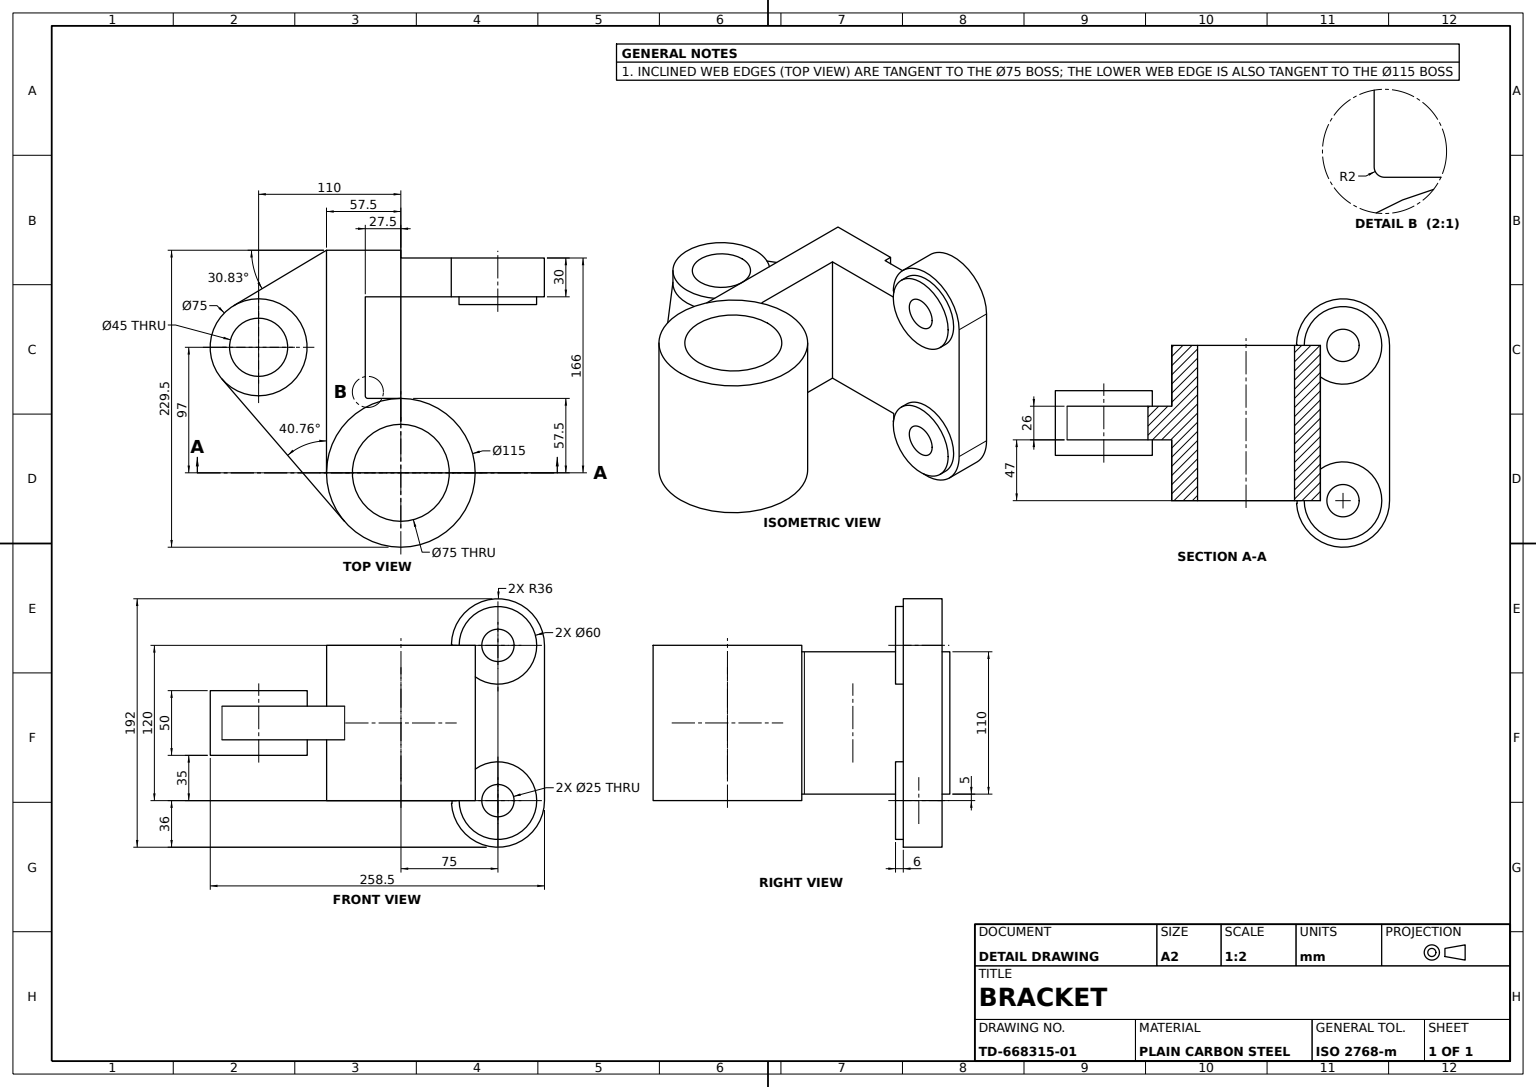
from build123d import *

# Parameters (mm, degrees)
BASE_PROFILE_SKETCH_R     = 12.5
BASE_BODY_DEPTH           = 15
BOSS_PAD_SKETCH_R         = 30
BOSS_PAD_6MM_DEPTH        = 6
BORE_SKETCH_R             = 12.5
BORE_CUT_DEPTH            = 145.976722269
ARM_BLOCK_SKETCH_R        = 57.5
ARM_BLOCK_SKETCH_R_2      = 37.5
ARM_BLOCK_DEPTH           = 60
WEB_DEPTH                 = 55
WEB_POCKET_SKETCH_W       = 39.351063387
WEB_POCKET_SKETCH_H       = 7.1816736
WEB_POCKET_SKETCH_W_2     = 45.776165888
WEB_POCKET_SKETCH_H_2     = 5.709571084
WEB_POCKET_CUT_DEPTH      = 97
MOUNTING_PLATE_SKETCH_R   = 37.5
MOUNTING_PLATE_SKETCH_R_2 = 22.5
MOUNTING_PLATE_DEPTH      = 25
LUG_BOSSES_DEPTH          = 13
LUG_HOLES_SKETCH_R        = 22.5
LUG_HOLES_CUT_DEPTH       = 329.05411139


with BuildPart() as part:
    # Base Profile Sketch → Base Body (new, symmetric)
    with BuildSketch(Plane.XY):
        with BuildLine():
            Line((-36, -60), (-102.5, -60))
            Line((-102.5, -60), (-102.5, 60))
            Line((-102.5, 60), (-36, 60))
            ThreePointArc((-36, 60), (0, 96), (36, 60))
            Line((36, 60), (36, -60))
            ThreePointArc((36, -60), (0, -96), (-36, -60))
        make_face()
        with Locations((0, 60)):
            Circle(BASE_PROFILE_SKETCH_R, mode=Mode.SUBTRACT)
        with Locations((0, -60)):
            Circle(BASE_PROFILE_SKETCH_R, mode=Mode.SUBTRACT)
    extrude(amount=BASE_BODY_DEPTH, both=True)

    # Boss Pad Sketch → Boss Pad 6mm (add)
    with BuildSketch(Plane.XY.offset(15)):
        with Locations((0, -60)):
            Circle(BOSS_PAD_SKETCH_R)
        with Locations((0, 60)):
            Circle(BOSS_PAD_SKETCH_R)
    extrude(amount=BOSS_PAD_6MM_DEPTH)

    # Bore Sketch → Bore Cut (cut, through all)
    with BuildSketch(Plane(origin=(0, 0, -15), x_dir=(-1, 0, 0), z_dir=(0, 0, -1))):
        with Locations((0, -60)):
            Circle(BORE_SKETCH_R)
        with Locations((0, 60)):
            Circle(BORE_SKETCH_R)
    extrude(amount=-BORE_CUT_DEPTH, mode=Mode.SUBTRACT)



with BuildPart() as body_2:
    # Arm Block Sketch → Arm Block (new, symmetric)
    with BuildSketch(Plane(origin=(0, 0, 0), x_dir=(1, 0, 0), z_dir=(0, 1, 0))):
        with Locations(Location((-75, -151, 0), (0, 0, 270))):
            Circle(ARM_BLOCK_SKETCH_R)
        with Locations(Location((-75, -151, 0), (0, 0, 270))):
            Circle(ARM_BLOCK_SKETCH_R_2, mode=Mode.SUBTRACT)
    extrude(amount=ARM_BLOCK_DEPTH, both=True)


with BuildPart() as part_1:
    add(part.part)

    add(body_2.part)  # Web merges body 2
    # Web Profile Sketch → Web (add, symmetric)
    with BuildSketch(Plane(origin=(0, 0, 0), x_dir=(1, 0, 0), z_dir=(0, 1, 0))):
        with BuildLine():
            Line((-132.5, -151), (-132.5, 21))
            Line((-132.5, 21), (-75, 21))
            Line((-75, 21), (-75, 15))
            Line((-75, 15), (-36, 15))
            Line((-36, 15), (-36, -15))
            Line((-36, -15), (-102.5, -15))
            Line((-102.5, -15), (-102.5, -91.5))
            ThreePointArc((-102.5, -91.5), (-101.914213562, -92.914213562), (-100.5, -93.5))
            Line((-100.5, -93.5), (-75, -93.5))
            ThreePointArc((-75, -93.5), (-115.658639918, -110.341360082), (-132.5, -151))
        make_face()
    extrude(amount=WEB_DEPTH, both=True)

    # Web Pocket Sketch → Web Pocket Cut (cut)
    with BuildSketch(Plane.ZY.offset(132.5)):
        with Locations((-1.324468307, -58.5908368)):
            Rectangle(WEB_POCKET_SKETCH_W, WEB_POCKET_SKETCH_H)
        with Locations((1.888082944, 57.854785542)):
            Rectangle(WEB_POCKET_SKETCH_W_2, WEB_POCKET_SKETCH_H_2)
    extrude(amount=-WEB_POCKET_CUT_DEPTH, mode=Mode.SUBTRACT)



with BuildPart() as body_2_2:
    # Mounting Plate Sketch → Mounting Plate (new, symmetric)
    with BuildSketch(Plane(origin=(0, 0, 0), x_dir=(1, 0, 0), z_dir=(0, 1, 0))):
        with Locations(Location((-185, -54, 0), (0, 0, 270))):
            Circle(MOUNTING_PLATE_SKETCH_R)
        with Locations(Location((-185, -54, 0), (0, 0, 270))):
            Circle(MOUNTING_PLATE_SKETCH_R_2, mode=Mode.SUBTRACT)
    extrude(amount=MOUNTING_PLATE_DEPTH, both=True)


with BuildPart() as part_2:
    add(part_1.part)

    add(body_2_2.part)  # Lug Bosses merges body 2 2
    # Lug Bosses Sketch → Lug Bosses (add, symmetric)
    with BuildSketch(Plane(origin=(0, 0, 0), x_dir=(1, 0, 0), z_dir=(0, 1, 0))):
        with BuildLine():
            Line((-132.5, 21), (-204.216934712, -21.798145701))
            ThreePointArc((-204.216934712, -21.798145701), (-222.016718342, -47.998953157), (-213.406251821, -78.481316498))
            Line((-213.406251821, -78.481316498), (-118.556252792, -188.53801863))
            Line((-118.556252792, -188.53801863), (-118.556252792, 21))
            Line((-118.556252792, 21), (-132.5, 21))
        make_face()
    extrude(amount=LUG_BOSSES_DEPTH, both=True)

    # Lug Holes Sketch → Lug Holes Cut (cut, through all)
    with BuildSketch(Plane.XZ.offset(25)):
        with Locations(Location((-185, 54, 0), (0, 0, 90))):
            Circle(LUG_HOLES_SKETCH_R)
    extrude(amount=-LUG_HOLES_CUT_DEPTH, mode=Mode.SUBTRACT)


solid = part_2.part
